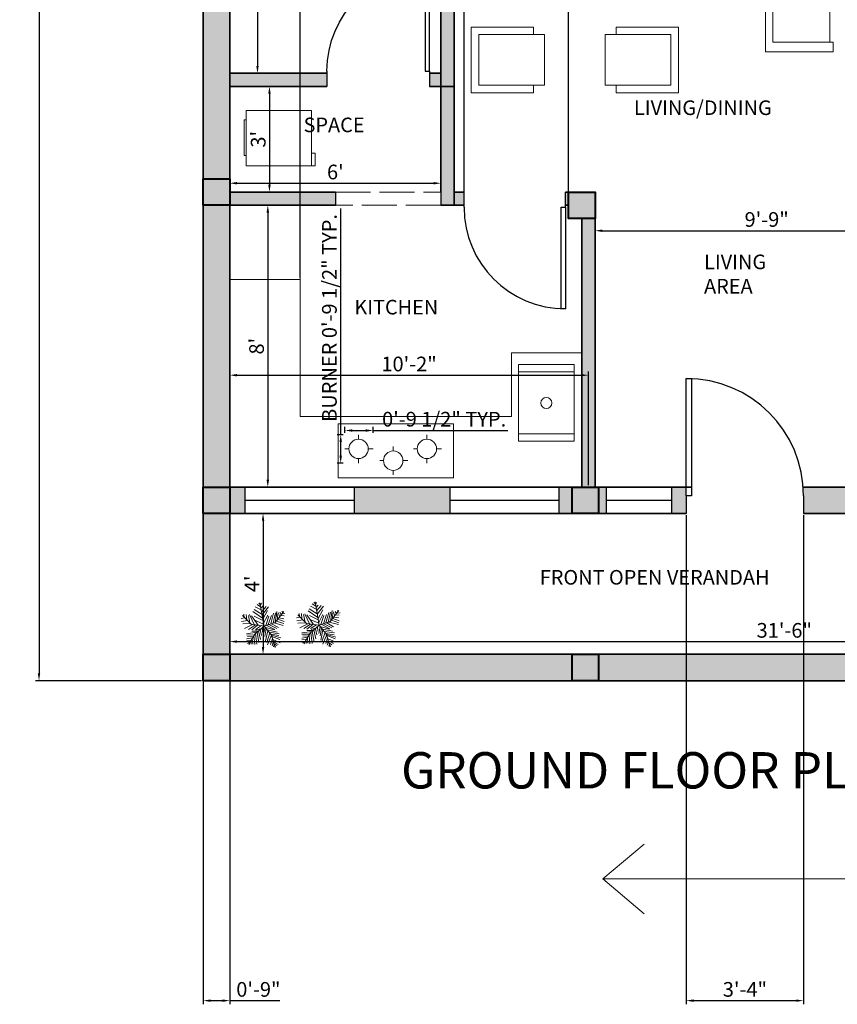
# Model space of a CAD drawing. Units: inches. Extents: x 1674 to 2231, y 1328 to 1959.
# Tile 1 of 6: x 1674 to 1952, y 1328 to 1664. Entities that reach past the tile are written whole.
import ezdxf

# ---------------------------------------------------------------- set-up
doc = ezdxf.new("R2010")
doc.units = ezdxf.units.IN
doc.linetypes.add('ACAD_ISO02W100', pattern=[15, 12, -3])
for name, color, linetype, lineweight in [('A-ANNO-DIMS', 113, 'Continuous', 18), ('A-ANNO-SYMB', 113, 'Continuous', 18), ('A-ANNO-TEXT', 113, 'Continuous', 18), ('A-AREA-IDEN', 113, 'Continuous', 18), ('A-COLS-PATT', 10, 'Continuous', 13), ('A-EQPM', 211, 'Continuous', 18), ('A-FLOR-CASE', 211, 'Continuous', 18), ('A-FLOR-FIXT', 211, 'Continuous', 18), ('A-GLAZ-HIDN', 181, 'ACAD_ISO02W100', 18), ('A-WALL-PATT', 140, 'Continuous', 13), ('COLUMN', 10, 'Continuous', 40), ('DOOR', 54, 'Continuous', 25), ('FUR', 211, 'Continuous', 18), ('TREE', 102, 'Continuous', 13), ('WALL', 7, 'Continuous', 35), ('WN', 181, 'Continuous', 25)]:
    doc.layers.add(name, color=color, linetype=linetype, lineweight=lineweight)
doc.styles.get("Standard").update_dxf_attribs({"font": 'arial.ttf'})
doc.dimstyles.new('ISO-25', dxfattribs={"dimtxt": 5, "dimasz": 2.5, "dimexe": 1.25, "dimexo": 0.625, "dimtad": 1, "dimdec": 0, "dimlunit": 4, "dimtxsty": 'Standard', "dimcen": 2.5, "dimadec": 0, "dimazin": 0, "dimtfac": 1, "dimtdec": 0, "dimtmove": 0, "dimatfit": 3, "dimfxl": 1, "dimarcsym": 0})

# ---------------------------------------------------------------- blocks, each defined once
blk = doc.blocks.new('*U2')
for p, q in [((0, 0), (0, -6)), ((40, 0), (40, -6))]:
    blk.add_line(p, q)
blk.add_lwpolyline([(0, 0), (0, 40), (1.75, 40), (1.75, 0)], close=True)
blk.add_arc((0, 0), 40, 0, 90)
blk = doc.blocks.new('*U8')
for p, q in [((-8.737, 47.138), (-17.069, 52.711)), ((-10.186, 53.64), (-13.084, 55.962)), ((0, 0), (-10.5, 57)), ((-9.099, 51.782), (-6.563, 55.962)), ((-7.65, 43.423), (-2.578, 49.46)), ((-31.5, 4.5), (-52.5, 25.5)), ((-48.585, 21.131), (-49.309, 29.026)), ((-43.513, 28.561), (-42.427, 15.558)), ((-38.442, 26.239), (-34.819, 7.663)), ((-35.544, 28.097), (-24.314, 3.947)), ((-14.533, 2.09), (-30.834, 25.31)), ((-3.665, 19.273), (-27.574, 35.527)), ((-5.114, 28.097), (-24.676, 40.636)), ((-7.288, 39.707), (-21.778, 46.673)), ((-5.839, 35.992), (4.667, 48.067)), ((-5.114, 27.632), (10.463, 46.673)), ((-2.941, 16.486), (8.652, 37.85)), ((-1.129, 6.734), (9.014, 26.704)), ((3.942, 1.625), (11.187, 24.381)), ((10.101, 3.483), (17.708, 26.239)), ((16.259, 5.805), (23.142, 31.348)), ((22.055, 7.198), (27.489, 32.277)), ((27, 9), (48, 36)), ((27.127, 9.056), (31.112, 35.992)), ((31.836, 30.883), (32.561, 16.486)), ((35.096, 32.741), (37.27, 22.524)), ((38.719, 34.134), (41.979, 28.561)), ((40.53, 25.775), (48.862, 24.846)), ((43.791, 29.954), (51.036, 30.883)), ((44.153, 36.456), (45.239, 32.741)), ((-47.498, 19.737), (-55.83, 18.344)), ((-40.615, 13.7), (-55.105, 10.913)), ((-33.37, 6.269), (-52.207, 5.34)), ((-28.299, 3.483), (-47.86, -5.805)), ((-21.416, 3.018), (-38.079, -8.128)), ((0, 0), (-31.5, 4.5)), ((-15.982, 2.09), (-30.11, -9.521)), ((-24.314, 23.917), (-2.941, 13.7)), ((0, 0), (-22.5, -19.5)), ((-6.563, 1.161), (-21.416, -8.128)), ((-20.691, 13.7), (-1.129, 4.876)), ((0, 0), (27, 9)), ((0, 0), (18, -22.5)), ((6.478, 1.625), (26.04, -8.592)), ((11.187, 3.483), (30.749, -5.805)), ((18.07, 5.805), (35.096, -3.483)), ((24.229, 7.663), (46.688, 1.625)), ((29.662, 12.307), (48.137, 6.269)), ((33.285, 16.486), (48.862, 10.913)), ((36.183, 19.737), (48.137, 17.88)), ((-17.431, -15.094), (-42.789, -18.809)), ((-24.314, -21.596), (-42.427, -22.06)), ((-22.5, -19.5), (-37.5, -45)), ((-15.257, -12.772), (-30.11, -12.772)), ((-25.038, -23.918), (-22.865, -45.281)), ((-20.691, -18.345), (-17.793, -44.352)), ((-6.563, -5.805), (-19.967, -9.985)), ((-17.069, -15.094), (-12.721, -40.172)), ((-13.446, -11.378), (-8.737, -32.741)), ((-9.461, -8.592), (-6.201, -23.453)), ((-4.752, -3.483), (-3.665, -14.629)), ((2.493, -3.019), (-1.491, -20.202)), ((1.769, -2.555), (24.229, -9.521)), ((5.029, -6.27), (2.131, -25.775)), ((9.014, -11.378), (3.58, -35.992)), ((14.085, -16.951), (6.478, -40.172)), ((7.565, -9.056), (32.198, -14.629)), ((18.07, -22.524), (8.289, -45.745)), ((12.274, -15.094), (36.907, -18.809)), ((16.259, -19.738), (36.183, -22.989)), ((18, -22.5), (27, -52.5)), ((18.433, -22.524), (40.53, -29.026)), ((-28.299, -29.026), (-42.789, -31.348)), ((-30.834, -34.135), (-42.427, -35.528)), ((-34.457, -39.708), (-40.978, -42.494)), ((-26.849, -26.24), (-40.253, -25.775)), ((-32.646, -36.921), (-31.921, -44.352)), ((-29.023, -30.884), (-27.936, -43.887)), ((20.244, -30.419), (15.897, -44.816)), ((19.157, -25.311), (38.719, -33.206)), ((22.78, -37.85), (19.519, -48.532)), ((21.331, -32.741), (39.081, -40.636)), ((22.78, -38.314), (34.372, -44.816)), ((24.591, -45.745), (23.142, -50.854)), ((24.591, -43.423), (30.749, -47.603)), ((26.764, -49.925), (28.213, -50.854))]:
    blk.add_line(p, q)
blk = doc.blocks.new('*D10')
at = {"layer": 'A-ANNO-DIMS', "color": 0, "lineweight": -2, "transparency": 16777216}
for p, q in [((1735.65, 1918.36), (1679.03, 1918.36)), ((1680.28, 1915.86), (1680.28, 1440.86)), ((1735.65, 1438.36), (1679.03, 1438.36))]:
    blk.add_line(p, q, dxfattribs=at)
at = {"layer": 'A-ANNO-DIMS', "color": 0, "lineweight": 100, "transparency": 16777216}
for points in [[(1679.86, 1915.86), (1680.69, 1915.86), (1680.28, 1918.36)], [(1679.86, 1440.86), (1680.69, 1440.86), (1680.28, 1438.36)]]:
    blk.add_solid(points, dxfattribs=at)
at = {"layer": 'Defpoints', "color": 0, "lineweight": 100, "transparency": 16777216}
for p in [(1736.27, 1918.36), (1680.28, 1438.36), (1736.27, 1438.36)]:
    blk.add_point(p, dxfattribs=at)
at = {"layer": 'A-ANNO-DIMS', "color": 0, "transparency": 16777216, "insert": (1677.1, 1678.36), "char_height": 5, "attachment_point": 5, "rotation": 90}
blk.add_mtext("40'", dxfattribs=at)
blk = doc.blocks.new('*D23')
at = {"layer": 'A-ANNO-DIMS', "color": 0, "lineweight": -2, "transparency": 16777216}
for p, q in [((1745.9, 1748.86), (1755.99, 1748.86)), ((1754.74, 1746.36), (1754.74, 1647.86)), ((1745.9, 1645.36), (1755.99, 1645.36))]:
    blk.add_line(p, q, dxfattribs=at)
at = {"layer": 'A-ANNO-DIMS', "color": 0, "lineweight": 100, "transparency": 16777216}
for points in [[(1754.32, 1746.36), (1755.15, 1746.36), (1754.74, 1748.86)], [(1754.32, 1647.86), (1755.15, 1647.86), (1754.74, 1645.36)]]:
    blk.add_solid(points, dxfattribs=at)
at = {"layer": 'Defpoints', "color": 0, "lineweight": 100, "transparency": 16777216}
for p in [(1745.27, 1748.86), (1745.27, 1645.36), (1754.74, 1645.36)]:
    blk.add_point(p, dxfattribs=at)
at = {"layer": 'A-ANNO-DIMS', "color": 0, "transparency": 16777216, "insert": (1751.56, 1697.11), "char_height": 5, "attachment_point": 5, "rotation": 90}
blk.add_mtext('8\'-8"', dxfattribs=at)
blk = doc.blocks.new('*D24')
at = {"layer": 'A-ANNO-DIMS', "color": 0, "lineweight": -2, "transparency": 16777216}
for p, q in [((1745.9, 1640.86), (1760.06, 1640.86)), ((1758.81, 1638.36), (1758.81, 1607.36)), ((1745.9, 1604.86), (1760.06, 1604.86))]:
    blk.add_line(p, q, dxfattribs=at)
at = {"layer": 'A-ANNO-DIMS', "color": 0, "lineweight": 100, "transparency": 16777216}
for points in [[(1758.39, 1638.36), (1759.23, 1638.36), (1758.81, 1640.86)], [(1758.39, 1607.36), (1759.23, 1607.36), (1758.81, 1604.86)]]:
    blk.add_solid(points, dxfattribs=at)
at = {"layer": 'Defpoints', "color": 0, "lineweight": 100, "transparency": 16777216}
for p in [(1745.27, 1640.86), (1745.27, 1604.86), (1758.81, 1604.86)]:
    blk.add_point(p, dxfattribs=at)
at = {"layer": 'A-ANNO-DIMS', "color": 0, "transparency": 16777216, "insert": (1755.63, 1622.86), "char_height": 5, "attachment_point": 5, "rotation": 90}
blk.add_mtext("3'", dxfattribs=at)
blk = doc.blocks.new('*D25')
at = {"layer": 'A-ANNO-DIMS', "color": 0, "lineweight": -2, "transparency": 16777216}
for p, q in [((1745.27, 1605.48), (1745.27, 1609.13)), ((1747.77, 1607.88), (1814.77, 1607.88)), ((1817.27, 1605.48), (1817.27, 1609.13))]:
    blk.add_line(p, q, dxfattribs=at)
at = {"layer": 'A-ANNO-DIMS', "color": 0, "lineweight": 100, "transparency": 16777216}
for points in [[(1747.77, 1608.3), (1747.77, 1607.46), (1745.27, 1607.88)], [(1814.77, 1608.3), (1814.77, 1607.46), (1817.27, 1607.88)]]:
    blk.add_solid(points, dxfattribs=at)
at = {"layer": 'Defpoints', "color": 0, "lineweight": 100, "transparency": 16777216}
for p in [(1817.27, 1607.88), (1745.27, 1604.86), (1817.27, 1604.86)]:
    blk.add_point(p, dxfattribs=at)
at = {"layer": 'A-ANNO-DIMS', "color": 0, "transparency": 16777216, "insert": (1781.27, 1611.06), "char_height": 5, "attachment_point": 5}
blk.add_mtext("6'", dxfattribs=at)
blk = doc.blocks.new('*D26')
at = {"layer": 'A-ANNO-DIMS', "color": 0, "lineweight": -2, "transparency": 16777216}
for p, q in [((1745.9, 1600.36), (1759.5, 1600.36)), ((1758.25, 1597.86), (1758.25, 1506.86)), ((1745.9, 1504.36), (1759.5, 1504.36))]:
    blk.add_line(p, q, dxfattribs=at)
at = {"layer": 'A-ANNO-DIMS', "color": 0, "lineweight": 100, "transparency": 16777216}
for points in [[(1757.83, 1597.86), (1758.67, 1597.86), (1758.25, 1600.36)], [(1757.83, 1506.86), (1758.67, 1506.86), (1758.25, 1504.36)]]:
    blk.add_solid(points, dxfattribs=at)
at = {"layer": 'Defpoints', "color": 0, "lineweight": 100, "transparency": 16777216}
for p in [(1745.27, 1600.36), (1745.27, 1504.36), (1758.25, 1504.36)]:
    blk.add_point(p, dxfattribs=at)
at = {"layer": 'A-ANNO-DIMS', "color": 0, "transparency": 16777216, "insert": (1755.07, 1552.36), "char_height": 5, "attachment_point": 5, "rotation": 90}
blk.add_mtext("8'", dxfattribs=at)
blk = doc.blocks.new('*D27')
at = {"layer": 'A-ANNO-DIMS', "color": 0, "lineweight": -2, "transparency": 16777216}
for p, q in [((1745.27, 1504.98), (1745.27, 1543.72)), ((1867.52, 1504.98), (1867.52, 1543.72)), ((1747.77, 1542.47), (1865.02, 1542.47))]:
    blk.add_line(p, q, dxfattribs=at)
at = {"layer": 'A-ANNO-DIMS', "color": 0, "lineweight": 100, "transparency": 16777216}
for points in [[(1747.77, 1542.88), (1747.77, 1542.05), (1745.27, 1542.47)], [(1865.02, 1542.88), (1865.02, 1542.05), (1867.52, 1542.47)]]:
    blk.add_solid(points, dxfattribs=at)
at = {"layer": 'Defpoints', "color": 0, "lineweight": 100, "transparency": 16777216}
for p in [(1867.52, 1542.47), (1745.27, 1504.36), (1867.52, 1504.36)]:
    blk.add_point(p, dxfattribs=at)
at = {"layer": 'A-ANNO-DIMS', "color": 0, "transparency": 16777216, "insert": (1806.4, 1545.64), "char_height": 5, "attachment_point": 5}
blk.add_mtext('10\'-2"', dxfattribs=at)
blk = doc.blocks.new('*D28')
at = {"layer": 'A-ANNO-DIMS', "color": 0, "lineweight": -2, "transparency": 16777216}
for p, q in [((1745.9, 1495.36), (1757.88, 1495.36)), ((1756.63, 1492.86), (1756.63, 1449.86)), ((1745.9, 1447.36), (1757.88, 1447.36))]:
    blk.add_line(p, q, dxfattribs=at)
at = {"layer": 'A-ANNO-DIMS', "color": 0, "lineweight": 100, "transparency": 16777216}
for points in [[(1756.22, 1492.86), (1757.05, 1492.86), (1756.63, 1495.36)], [(1756.22, 1449.86), (1757.05, 1449.86), (1756.63, 1447.36)]]:
    blk.add_solid(points, dxfattribs=at)
at = {"layer": 'Defpoints', "color": 0, "lineweight": 100, "transparency": 16777216}
for p in [(1745.27, 1495.36), (1745.27, 1447.36), (1756.63, 1447.36)]:
    blk.add_point(p, dxfattribs=at)
at = {"layer": 'A-ANNO-DIMS', "color": 0, "transparency": 16777216, "insert": (1753.51, 1471.36), "char_height": 5, "attachment_point": 5, "rotation": 90}
blk.add_mtext("4'", dxfattribs=at)
blk = doc.blocks.new('*D29')
at = {"layer": 'A-ANNO-DIMS', "color": 0, "lineweight": -2, "transparency": 16777216}
for p, q in [((1745.27, 1447.98), (1745.27, 1452.95)), ((2123.27, 1447.98), (2123.27, 1452.95)), ((1747.77, 1451.7), (2120.77, 1451.7))]:
    blk.add_line(p, q, dxfattribs=at)
at = {"layer": 'A-ANNO-DIMS', "color": 0, "lineweight": 100, "transparency": 16777216}
for points in [[(1747.77, 1452.12), (1747.77, 1451.28), (1745.27, 1451.7)], [(2120.77, 1452.12), (2120.77, 1451.28), (2123.27, 1451.7)]]:
    blk.add_solid(points, dxfattribs=at)
at = {"layer": 'Defpoints', "color": 0, "lineweight": 100, "transparency": 16777216}
for p in [(2123.27, 1451.7), (1745.27, 1447.36), (2123.27, 1447.36)]:
    blk.add_point(p, dxfattribs=at)
at = {"layer": 'A-ANNO-DIMS', "color": 0, "transparency": 16777216, "insert": (1934.27, 1454.88), "char_height": 5, "attachment_point": 5}
blk.add_mtext('31\'-6"', dxfattribs=at)
blk = doc.blocks.new('*D30')
at = {"layer": 'A-ANNO-DIMS', "color": 0, "lineweight": -2, "transparency": 16777216}
for p, q in [((1869.77, 1504.98), (1869.77, 1592.95)), ((1872.27, 1591.7), (1984.27, 1591.7)), ((1986.77, 1504.98), (1986.77, 1592.95))]:
    blk.add_line(p, q, dxfattribs=at)
at = {"layer": 'A-ANNO-DIMS', "color": 0, "lineweight": 100, "transparency": 16777216}
for points in [[(1872.27, 1592.11), (1872.27, 1591.28), (1869.77, 1591.7)], [(1984.27, 1592.11), (1984.27, 1591.28), (1986.77, 1591.7)]]:
    blk.add_solid(points, dxfattribs=at)
at = {"layer": 'Defpoints', "color": 0, "lineweight": 100, "transparency": 16777216}
for p in [(1986.77, 1591.7), (1869.77, 1504.36), (1986.77, 1504.36)]:
    blk.add_point(p, dxfattribs=at)
at = {"layer": 'A-ANNO-DIMS', "color": 0, "transparency": 16777216, "insert": (1928.27, 1594.88), "char_height": 5, "attachment_point": 5}
blk.add_mtext('9\'-9"', dxfattribs=at)
blk = doc.blocks.new('CHAIR-DINING')
for p, q in [((21.28, 22.31), (0, 22.31)), ((0, 22.31), (0, 0)), ((21.28, 19.89), (21.28, 22.31)), ((0, 0), (21.28, 0)), ((21.28, 0), (21.28, 2.58))]:
    blk.add_line(p, q)
blk.add_lwpolyline([(25.04, 19.89), (2.65, 19.89), (2.65, 2.58), (25.04, 2.58)], close=True)
blk = doc.blocks.new('ARROW-ROAD-DIRECTION')
for p, q in [((0, 11.86), (14.05, 23.72)), ((88.42, 11.86), (0, 11.86)), ((4.6, 11.86), (0, 11.86)), ((0, 11.86), (14.05, 0))]:
    blk.add_line(p, q)
blk = doc.blocks.new('COOKTOP-BURNER')
for p, q in [((4.62, 8.16), (4.62, 9.66)), ((1.32, 4.86), (0, 4.86)), ((7.93, 4.86), (9.61, 4.86)), ((4.62, 1.56), (4.62, 0))]:
    blk.add_line(p, q)
blk.add_circle((4.62, 4.86), 3.3)
blk = doc.blocks.new('*D44')
at = {"layer": 'A-ANNO-DIMS', "color": 0, "lineweight": -2, "transparency": 16777216}
for p, q in [((1783.1, 1522.17), (1783.1, 1599.27)), ((1783.92, 1522.17), (1781.85, 1522.17)), ((1783.1, 1515.01), (1783.1, 1519.67)), ((1783.92, 1512.51), (1781.85, 1512.51))]:
    blk.add_line(p, q, dxfattribs=at)
at = {"layer": 'A-ANNO-DIMS', "color": 0, "lineweight": 100, "transparency": 16777216}
for points in [[(1782.68, 1519.67), (1783.52, 1519.67), (1783.1, 1522.17)], [(1782.68, 1515.01), (1783.52, 1515.01), (1783.1, 1512.51)]]:
    blk.add_solid(points, dxfattribs=at)
at = {"layer": 'Defpoints', "color": 0, "lineweight": 100, "transparency": 16777216}
for p in [(1783.1, 1522.17), (1784.55, 1522.17), (1784.55, 1512.51)]:
    blk.add_point(p, dxfattribs=at)
at = {"layer": 'A-ANNO-DIMS', "color": 0, "transparency": 16777216, "insert": (1779.89, 1561.97), "char_height": 5, "attachment_point": 5, "rotation": 90}
blk.add_mtext('BURNER 0\'-9 1/2" TYP.', dxfattribs=at)
blk = doc.blocks.new('*D45')
at = {"layer": 'A-ANNO-DIMS', "color": 0, "lineweight": -2, "transparency": 16777216}
for p, q in [((1784.55, 1522.8), (1784.55, 1524.87)), ((1787.05, 1523.62), (1791.66, 1523.62)), ((1794.16, 1522.8), (1794.16, 1524.87)), ((1794.16, 1523.62), (1840.03, 1523.62))]:
    blk.add_line(p, q, dxfattribs=at)
at = {"layer": 'A-ANNO-DIMS', "color": 0, "lineweight": 100, "transparency": 16777216}
for points in [[(1787.05, 1524.04), (1787.05, 1523.21), (1784.55, 1523.62)], [(1791.66, 1524.04), (1791.66, 1523.21), (1794.16, 1523.62)]]:
    blk.add_solid(points, dxfattribs=at)
at = {"layer": 'Defpoints', "color": 0, "lineweight": 100, "transparency": 16777216}
for p in [(1794.16, 1523.62), (1784.55, 1522.17), (1794.16, 1522.17)]:
    blk.add_point(p, dxfattribs=at)
at = {"layer": 'A-ANNO-DIMS', "color": 0, "transparency": 16777216, "insert": (1818.35, 1526.83), "char_height": 5, "attachment_point": 5}
blk.add_mtext('0\'-9 1/2" TYP.', dxfattribs=at)
blk = doc.blocks.new('*D51')
at = {"layer": 'A-ANNO-DIMS', "color": 0, "lineweight": -2, "transparency": 16777216}
for p, q in [((1900.85, 1494.73), (1900.85, 1328.11)), ((1940.85, 1494.73), (1940.85, 1328.11)), ((1903.35, 1329.36), (1938.35, 1329.36))]:
    blk.add_line(p, q, dxfattribs=at)
at = {"layer": 'A-ANNO-DIMS', "color": 0, "lineweight": 100, "transparency": 16777216}
for points in [[(1903.35, 1329.77), (1903.35, 1328.94), (1900.85, 1329.36)], [(1938.35, 1329.77), (1938.35, 1328.94), (1940.85, 1329.36)]]:
    blk.add_solid(points, dxfattribs=at)
at = {"layer": 'Defpoints', "color": 0, "lineweight": 100, "transparency": 16777216}
for p in [(1900.85, 1495.36), (1940.85, 1495.36), (1940.85, 1329.36)]:
    blk.add_point(p, dxfattribs=at)
at = {"layer": 'A-ANNO-DIMS', "color": 0, "transparency": 16777216, "insert": (1920.85, 1332.54), "char_height": 5, "attachment_point": 5}
blk.add_mtext('3\'-4"', dxfattribs=at)
blk = doc.blocks.new('*D54')
at = {"layer": 'A-ANNO-DIMS', "color": 0, "lineweight": -2, "transparency": 16777216}
for p, q in [((1745.27, 1575.73), (1745.27, 1949.21)), ((1747.77, 1947.96), (1766.77, 1947.96)), ((1769.27, 1575.73), (1769.27, 1949.21))]:
    blk.add_line(p, q, dxfattribs=at)
at = {"layer": 'A-ANNO-DIMS', "color": 0, "lineweight": 100, "transparency": 16777216}
for points in [[(1747.77, 1948.37), (1747.77, 1947.54), (1745.27, 1947.96)], [(1766.77, 1948.37), (1766.77, 1947.54), (1769.27, 1947.96)]]:
    blk.add_solid(points, dxfattribs=at)
at = {"layer": 'Defpoints', "color": 0, "lineweight": 100, "transparency": 16777216}
for p in [(1769.27, 1947.96), (1745.27, 1575.1), (1769.27, 1575.1)]:
    blk.add_point(p, dxfattribs=at)
at = {"layer": 'A-ANNO-DIMS', "color": 0, "transparency": 16777216, "insert": (1757.27, 1951.13), "char_height": 5, "attachment_point": 5}
blk.add_mtext('2\'-0"', dxfattribs=at)
blk = doc.blocks.new('*D55')
at = {"layer": 'A-ANNO-DIMS', "color": 0, "lineweight": -2, "transparency": 16777216}
for p, q in [((1736.27, 1494.73), (1736.27, 1328.11)), ((1745.27, 1494.73), (1745.27, 1328.11)), ((1738.77, 1329.36), (1742.77, 1329.36)), ((1745.27, 1329.36), (1762.31, 1329.36))]:
    blk.add_line(p, q, dxfattribs=at)
at = {"layer": 'A-ANNO-DIMS', "color": 0, "lineweight": 100, "transparency": 16777216}
for points in [[(1738.77, 1329.77), (1738.77, 1328.94), (1736.27, 1329.36)], [(1742.77, 1329.77), (1742.77, 1328.94), (1745.27, 1329.36)]]:
    blk.add_solid(points, dxfattribs=at)
at = {"layer": 'Defpoints', "color": 0, "lineweight": 100, "transparency": 16777216}
for p in [(1736.27, 1495.36), (1745.27, 1495.36), (1745.27, 1329.36)]:
    blk.add_point(p, dxfattribs=at)
at = {"layer": 'A-ANNO-DIMS', "color": 0, "transparency": 16777216, "insert": (1755.04, 1332.54), "char_height": 5, "attachment_point": 5}
blk.add_mtext('0\'-9"', dxfattribs=at)
blk = doc.blocks.new('*D56')
at = {"layer": 'A-ANNO-DIMS', "color": 0, "lineweight": -2, "transparency": 16777216}
for p, q in [((1825.14, 1600.98), (1825.14, 1949.21)), ((1827.64, 1947.96), (1858.27, 1947.96)), ((1860.77, 1600.98), (1860.77, 1949.21))]:
    blk.add_line(p, q, dxfattribs=at)
at = {"layer": 'A-ANNO-DIMS', "color": 0, "lineweight": 100, "transparency": 16777216}
for points in [[(1827.64, 1948.37), (1827.64, 1947.54), (1825.14, 1947.96)], [(1858.27, 1948.37), (1858.27, 1947.54), (1860.77, 1947.96)]]:
    blk.add_solid(points, dxfattribs=at)
at = {"layer": 'Defpoints', "color": 0, "lineweight": 100, "transparency": 16777216}
for p in [(1860.77, 1947.96), (1825.14, 1600.36), (1860.77, 1600.36)]:
    blk.add_point(p, dxfattribs=at)
at = {"layer": 'A-ANNO-DIMS', "color": 0, "transparency": 16777216, "insert": (1842.96, 1951.17), "char_height": 5, "attachment_point": 5}
blk.add_mtext('2\'-11 1/2"', dxfattribs=at)

msp = doc.modelspace()

# ---------------------------------------------------------------- hatches: boundary and pattern name
at = {"layer": 'A-COLS-PATT'}
h = msp.add_hatch(color=256, dxfattribs=at)
h.dxf.hatch_style = 1
h.paths.add_polyline_path([(1745.27, 1918.36), (1736.27, 1918.36), (1736.27, 1909.36), (1745.27, 1909.36)])
h.paths.add_polyline_path([(1886.27, 1918.36), (1877.27, 1918.36), (1877.27, 1909.36), (1886.27, 1909.36)])
h.paths.add_polyline_path([(1995.77, 1918.36), (1986.77, 1918.36), (1986.77, 1909.36), (1995.77, 1909.36)])
h.paths.add_polyline_path([(2132.27, 1918.36), (2123.27, 1918.36), (2123.27, 1909.36), (2132.27, 1909.36)])
h.paths.add_polyline_path([(1745.27, 1757.86), (1736.27, 1757.86), (1736.27, 1748.86), (1745.27, 1748.86)])
h.paths.add_polyline_path([(1886.27, 1757.86), (1877.27, 1757.86), (1877.27, 1748.86), (1886.27, 1748.86)])
h.paths.add_polyline_path([(2132.27, 1757.81), (2123.27, 1757.81), (2123.27, 1748.81), (2132.27, 1748.81)])
h.paths.add_polyline_path([(1995.77, 1757.86), (1986.77, 1757.86), (1986.77, 1748.86), (1995.77, 1748.86)])
h.paths.add_polyline_path([(2132.27, 1625.36), (2123.27, 1625.36), (2123.27, 1616.36), (2132.27, 1616.36)])
h.paths.add_polyline_path([(1995.77, 1625.36), (1986.77, 1625.36), (1986.77, 1616.36), (1995.77, 1616.36)])
h.paths.add_polyline_path([(1869.77, 1604.86), (1860.77, 1604.86), (1860.77, 1595.86), (1869.77, 1595.86)])
h.paths.add_polyline_path([(1745.27, 1609.36), (1736.27, 1609.36), (1736.27, 1600.36), (1745.27, 1600.36)])
h.paths.add_polyline_path([(1745.27, 1504.36), (1736.27, 1504.36), (1736.27, 1495.36), (1745.27, 1495.36)])
h.paths.add_polyline_path([(1870.95, 1504.36), (1861.95, 1504.36), (1861.95, 1495.36), (1870.95, 1495.36)])
h.paths.add_polyline_path([(1995.77, 1504.36), (1986.77, 1504.36), (1986.77, 1495.36), (1995.77, 1495.36)])
h.paths.add_polyline_path([(1995.77, 1447.36), (1986.77, 1447.36), (1986.77, 1438.36), (1995.77, 1438.36)])
h.paths.add_polyline_path([(2132.27, 1447.36), (2123.27, 1447.36), (2123.27, 1438.36), (2132.27, 1438.36)])
h = msp.add_hatch(color=256, dxfattribs=at)
h.dxf.hatch_style = 1
h.paths.add_polyline_path([(1745.27, 1447.36), (1736.27, 1447.36), (1736.27, 1438.36), (1745.27, 1438.36)])
h.paths.add_polyline_path([(1870.95, 1447.36), (1861.95, 1447.36), (1861.95, 1438.36), (1870.95, 1438.36)])
at = {"layer": 'A-WALL-PATT'}
h = msp.add_hatch(color=256, dxfattribs=at)
h.dxf.hatch_style = 1
h.paths.add_polyline_path([(1877.27, 1918.36), (1745.27, 1918.36), (1745.27, 1909.36), (1877.27, 1909.36)])
h.paths.add_polyline_path([(1986.77, 1918.36), (1886.27, 1918.36), (1886.27, 1909.36), (1986.77, 1909.36)])
h.paths.add_polyline_path([(2123.27, 1918.36), (1995.77, 1918.36), (1995.77, 1909.36), (2123.27, 1909.36)])
h.paths.add_polyline_path([(1894.11, 1861.36), (1886.27, 1861.36), (1886.27, 1865.74), (1881.77, 1865.74), (1881.77, 1808), (1881.77, 1798.89), (1884.87, 1798.89, -0.017002), (1886.27, 1798.84), (1886.27, 1852.36), (1894.11, 1852.36)])
h.paths.add_polyline_path([(1952.87, 1861.36), (1919.24, 1861.36), (1919.24, 1852.36), (1952.87, 1852.36)])
h.paths.add_polyline_path([(1991.27, 1865.74), (1986.77, 1865.74), (1986.77, 1861.36), (1976.26, 1861.36), (1976.26, 1852.36), (1986.77, 1852.36), (1986.77, 1847.49), (1986.77, 1757.86), (1991.27, 1757.86), (1991.27, 1852.36)])
h.paths.add_polyline_path([(1986.77, 1816.36), (1938.77, 1816.36), (1938.77, 1813.86), (1986.77, 1813.86)])
h.paths.add_polyline_path([(1934.27, 1819.36), (1886.27, 1819.36), (1886.27, 1816.86), (1934.27, 1816.86)])
h.paths.add_polyline_path([(1938.77, 1852.36), (1934.27, 1852.36), (1934.27, 1753.36), (1934.27, 1748.86), (1938.77, 1748.86), (1938.77, 1753.36)])
h.paths.add_polyline_path([(1934.27, 1777.36), (1915.46, 1777.36), (1886.27, 1777.36), (1886.27, 1772.86), (1934.27, 1772.86)])
h.paths.add_polyline_path([(1986.77, 1753.36), (1967.96, 1753.36), (1961.77, 1753.36, -0.017002), (1961.81, 1751.95), (1961.81, 1748.86), (1986.77, 1748.86)])
h.paths.add_polyline_path([(2000.84, 1753.36), (1995.77, 1753.36), (1995.77, 1748.86), (2000.84, 1748.86)])
h.paths.add_polyline_path([(1941.17, 1751.95), (1941.17, 1753.36), (1938.77, 1753.36), (1938.77, 1748.86), (1941.17, 1748.86)])
h.paths.add_polyline_path([(1877.27, 1753.36), (1875.49, 1753.36), (1875.49, 1748.86), (1877.27, 1748.86)])
h.paths.add_polyline_path([(1745.27, 1909.36), (1736.27, 1909.36), (1736.27, 1757.86), (1745.27, 1757.86), (1745.27, 1773.01)])
h.paths.add_polyline_path([(1778.41, 1645.36), (1745.27, 1645.36), (1745.27, 1640.86), (1778.41, 1640.86)])
h.paths.add_polyline_path([(1821.77, 1645.36), (1821.77, 1668.45), (1817.27, 1668.45), (1817.27, 1645.36), (1817.27, 1640.86), (1821.77, 1640.86)])
h.paths.add_polyline_path([(1817.27, 1645.36), (1813.39, 1645.36), (1813.39, 1640.86), (1817.27, 1640.86)])
h.paths.add_polyline_path([(1821.77, 1640.86), (1817.27, 1640.86), (1817.27, 1604.86), (1817.27, 1600.36), (1821.77, 1600.36)])
h.paths.add_polyline_path([(1825.14, 1604.86), (1821.77, 1604.86), (1821.77, 1600.36), (1825.14, 1600.36)])
h.paths.add_polyline_path([(1781.27, 1604.86), (1745.27, 1604.86), (1745.27, 1600.36), (1781.27, 1600.36)])
h = msp.add_hatch(color=256, dxfattribs=at)
h.dxf.hatch_style = 1
h.paths.add_polyline_path([(2132.27, 1909.36), (2123.27, 1909.36), (2123.27, 1757.81), (2132.27, 1757.81)], flags=17)
h.paths.add_polyline_path([(2123.27, 1753.36), (2040.84, 1753.36), (2040.84, 1748.86), (2123.27, 1748.86)], flags=17)
h.paths.add_polyline_path([(1840.51, 1753.36), (1745.27, 1753.36), (1745.27, 1748.86), (1817.27, 1748.86), (1840.51, 1748.86)], flags=17)
h.paths.add_polyline_path([(1745.27, 1748.86), (1736.27, 1748.86), (1736.27, 1609.36), (1745.27, 1609.36), (1745.27, 1640.86)], flags=17)
h.paths.add_polyline_path([(1745.27, 1600.36), (1736.27, 1600.36), (1736.27, 1504.36), (1745.27, 1504.36)], flags=17)
h.paths.add_polyline_path([(1745.27, 1495.36), (1736.27, 1495.36), (1736.27, 1447.36), (1745.27, 1447.36)], flags=17)
h.paths.add_polyline_path([(1820.35, 1504.36), (1787.69, 1504.36), (1787.69, 1495.36), (1820.35, 1495.36)], flags=17)
h.paths.add_polyline_path([(1750.58, 1504.36), (1745.27, 1504.36), (1745.27, 1495.36), (1750.58, 1495.36)], flags=17)
h.paths.add_polyline_path([(1861.95, 1504.36), (1857.47, 1504.36), (1857.47, 1495.36), (1861.95, 1495.36)], flags=17)
h.paths.add_polyline_path([(1873.66, 1504.36), (1870.95, 1504.36), (1870.95, 1495.36), (1873.66, 1495.36)], flags=17)
h.paths.add_polyline_path([(1900.85, 1501.36), (1900.85, 1504.36), (1895.88, 1504.36), (1895.88, 1495.36), (1900.85, 1495.36)], flags=17)
h.paths.add_polyline_path([(1869.77, 1595.86), (1865.27, 1595.86), (1865.27, 1504.36), (1869.77, 1504.36)], flags=17)
h.paths.add_polyline_path([(1958.26, 1504.36), (1940.74, 1504.36, -0.01877), (1940.85, 1501.36), (1940.85, 1495.36), (1958.26, 1495.36)], flags=17)
h.paths.add_polyline_path([(1995.77, 1531.51), (1986.77, 1531.51), (1986.77, 1504.36), (1995.77, 1504.36)], flags=17)
h.paths.add_polyline_path([(1986.77, 1504.36), (1980.49, 1504.36), (1980.49, 1495.36), (1986.77, 1495.36)], flags=17)
h.paths.add_polyline_path([(1995.77, 1616.36), (1986.77, 1616.36), (1986.77, 1585.02), (1995.77, 1585.02)], flags=17)
h.paths.add_polyline_path([(2000.1, 1620.86), (1995.77, 1620.86), (1995.77, 1616.36), (2000.1, 1616.36)], flags=17)
h.paths.add_polyline_path([(2053.57, 1620.86), (2040.1, 1620.86), (2040.1, 1616.36), (2053.57, 1616.36)], flags=17)
h.paths.add_polyline_path([(2123.27, 1620.86), (2109.12, 1620.86), (2109.12, 1616.36), (2123.27, 1616.36)], flags=17)
h.paths.add_polyline_path([(2132.27, 1616.36), (2123.27, 1616.36), (2123.27, 1447.36), (2132.27, 1447.36)], flags=17)
h.paths.add_polyline_path([(1986.77, 1447.36), (1870.95, 1447.36), (1870.95, 1438.36), (1986.77, 1438.36)])
h.paths.add_polyline_path([(1861.95, 1447.36), (1745.27, 1447.36), (1745.27, 1438.36), (1861.95, 1438.36)])
h.paths.add_polyline_path([(2132.27, 1918.36), (1736.27, 1918.36), (1736.27, 1504.36), (1745.27, 1504.36), (1745.27, 1600.36), (1745.27, 1909.36), (2123.27, 1909.36), (2123.27, 1447.36), (2132.27, 1447.36)])
h = msp.add_hatch(color=256, dxfattribs=at)
h.dxf.hatch_style = 1
h.paths.add_polyline_path([(1745.27, 1600.36), (1736.27, 1600.36), (1736.27, 1504.36), (1745.27, 1504.36)])
h.paths.add_polyline_path([(1745.27, 1748.86), (1736.27, 1748.86), (1736.27, 1609.36), (1745.27, 1609.36), (1745.27, 1640.86)])
h.paths.add_polyline_path([(1821.77, 1748.86), (1817.27, 1748.86), (1817.27, 1723.23), (1821.77, 1723.23)])
h = msp.add_hatch(color=256, dxfattribs=at)
h.dxf.hatch_style = 1
h.paths.add_polyline_path([(1860.77, 1604.86), (1859.69, 1604.86), (1859.69, 1600.36), (1860.77, 1600.36)])

# ---------------------------------------------------------------- linework, layer by layer
at = {"layer": 'A-EQPM'}
for points in [[(1750.89, 1613.84), (1773.12, 1613.84), (1773.12, 1632.67), (1750.89, 1632.67)], [(1750.89, 1617.35), (1750.19, 1617.35), (1750.19, 1629.54), (1750.89, 1629.54)], [(1773.12, 1613.84), (1774.35, 1613.84), (1774.35, 1618.11), (1773.12, 1618.11)], [(1782.24, 1525.86), (1821.49, 1525.86), (1821.49, 1507.55), (1782.24, 1507.55)]]:
    msp.add_lwpolyline(points, close=True, dxfattribs=at)
at = {"layer": 'A-FLOR-CASE'}
for p, q in [((1745.27, 1600.36), (1769.27, 1600.36)), ((1769.27, 1600.36), (1769.27, 1528.36)), ((1865.27, 1550.11), (1841.27, 1550.11)), ((1841.27, 1550.11), (1841.27, 1528.36)), ((1841.27, 1528.36), (1769.27, 1528.36))]:
    msp.add_line(p, q, dxfattribs=at)
msp.add_lwpolyline([(1745.27, 1600.36), (1769.27, 1600.36), (1769.27, 1575.1), (1745.27, 1575.1)], close=True, dxfattribs=at)
at = {"layer": 'A-FLOR-FIXT'}
for p, q in [((1843.74, 1543.6), (1862.66, 1543.6)), ((1843.74, 1522.51), (1862.66, 1522.51))]:
    msp.add_line(p, q, dxfattribs=at)
msp.add_lwpolyline([(1843.74, 1546.09), (1862.66, 1546.09), (1862.66, 1519.94), (1843.74, 1519.94)], close=True, dxfattribs=at)
msp.add_circle((1853.2, 1533.01), 1.89, dxfattribs=at)
at = {"layer": 'A-GLAZ-HIDN'}
msp.add_lwpolyline([(1817.27, 1600.36), (1781.27, 1600.36), (1781.27, 1604.86), (1817.27, 1604.86)], close=True, dxfattribs=at)
at = {"layer": 'COLUMN'}
for points in [[(1736.27, 1609.36), (1745.27, 1609.36), (1745.27, 1600.36), (1736.27, 1600.36)], [(1860.77, 1604.86), (1869.77, 1604.86), (1869.77, 1595.86), (1860.77, 1595.86)], [(1736.27, 1504.36), (1745.27, 1504.36), (1745.27, 1495.36), (1736.27, 1495.36)], [(1861.95, 1504.36), (1870.95, 1504.36), (1870.95, 1495.36), (1861.95, 1495.36)], [(1736.27, 1447.36), (1745.27, 1447.36), (1745.27, 1438.36), (1736.27, 1438.36)], [(1861.95, 1447.36), (1870.95, 1447.36), (1870.95, 1438.36), (1861.95, 1438.36)]]:
    msp.add_lwpolyline(points, close=True, dxfattribs=at)
at = {"layer": 'FUR'}
for p, q in [((1927.85, 1652.61), (1927.85, 1720.04)), ((1949.77, 1655.93), (1950.89, 1655.93)), ((1950.89, 1655.93), (1950.89, 1652.61)), ((1950.89, 1652.61), (1927.85, 1652.61))]:
    msp.add_line(p, q, dxfattribs=at)
msp.add_lwpolyline([(1930.34, 1717.22), (1949.77, 1717.22), (1949.77, 1655.93), (1930.34, 1655.93)], close=True, dxfattribs=at)
at = {"layer": 'WALL'}
for p, q in [((1736.27, 1438.36), (1736.27, 1918.36)), ((1817.27, 1748.86), (1817.27, 1645.36)), ((1821.77, 1748.86), (1821.77, 1640.86)), ((1778.41, 1645.36), (1745.27, 1645.36)), ((1817.27, 1645.36), (1813.39, 1645.36)), ((1817.27, 1604.86), (1817.27, 1645.36)), ((1821.77, 1600.36), (1821.77, 1645.36)), ((1745.27, 1640.86), (1745.27, 1604.86)), ((1778.41, 1640.86), (1745.27, 1640.86)), ((1821.77, 1640.86), (1813.39, 1640.86)), ((1745.27, 1604.86), (1781.27, 1604.86)), ((1825.14, 1604.86), (1821.77, 1604.86)), ((1869.77, 1604.86), (1859.69, 1604.86)), ((1869.77, 1504.36), (1869.77, 1604.86)), ((1745.27, 1600.36), (1781.27, 1600.36)), ((1745.27, 1600.36), (1745.27, 1504.36)), ((1817.27, 1600.36), (1821.77, 1600.36)), ((1825.14, 1600.36), (1821.77, 1600.36)), ((1860.77, 1600.36), (1859.69, 1600.36)), ((1865.27, 1504.36), (1865.27, 1595.86)), ((1745.27, 1504.36), (1865.27, 1504.36)), ((1865.27, 1504.36), (1869.77, 1504.36)), ((1869.77, 1504.36), (1902.6, 1504.36)), ((1940.74, 1504.36), (1986.77, 1504.36)), ((1745.27, 1495.36), (1869.77, 1495.36)), ((1869.77, 1495.36), (1900.85, 1495.36)), ((1940.85, 1495.36), (1995.77, 1495.36)), ((1995.77, 1438.36), (1736.27, 1438.36))]:
    msp.add_line(p, q, dxfattribs=at)
for points in [[(1995.77, 1438.36), (1736.27, 1438.36), (1736.27, 1918.36), (2132.27, 1918.36), (2132.27, 1438.36), (2123.27, 1438.36)], [(1995.77, 1447.36), (1745.27, 1447.36), (1745.27, 1909.36), (2123.27, 1909.36), (2123.27, 1447.36)]]:
    msp.add_lwpolyline(points, dxfattribs=at)
at = {"layer": 'WN'}
for p, q in [((1781.27, 1604.86), (1781.27, 1600.36)), ((1817.27, 1604.86), (1817.27, 1600.36)), ((1750.58, 1499.86), (1787.69, 1499.86)), ((1820.35, 1499.86), (1857.47, 1499.86)), ((1873.66, 1499.86), (1895.88, 1499.86))]:
    msp.add_line(p, q, dxfattribs=at)
for points in [[(1750.58, 1504.36), (1787.69, 1504.36), (1787.69, 1495.36), (1750.58, 1495.36)], [(1820.35, 1504.36), (1857.47, 1504.36), (1857.47, 1495.36), (1820.35, 1495.36)], [(1873.66, 1504.36), (1895.88, 1504.36), (1895.88, 1495.36), (1873.66, 1495.36)]]:
    msp.add_lwpolyline(points, close=True, dxfattribs=at)

# ---------------------------------------------------------------- block references
at = {"layer": 'A-ANNO-SYMB'}
msp.add_blockref('ARROW-ROAD-DIRECTION', (1872.46, 1358.96), dxfattribs=at)
at = {"layer": 'A-EQPM'}
for p in [(1784.55, 1512.51), (1807.85, 1512.51), (1796.38, 1508.49)]:
    msp.add_blockref('COOKTOP-BURNER', p, dxfattribs=at)
at = {"layer": 'DOOR', "xscale": -0.8744829560094038, "yscale": 0.8744829560094038, "zscale": 0.8744829560094038}
msp.add_blockref('*U2', (1813.39, 1646.1), dxfattribs=at)
at = {"layer": 'DOOR', "xscale": 0.863878905869771, "yscale": 0.863878905869771, "zscale": 0.863878905869771, "rotation": 180}
msp.add_blockref('*U2', (1859.69, 1599.67), dxfattribs=at)
at = {"layer": 'DOOR'}
msp.add_blockref('*U2', (1900.85, 1501.36), dxfattribs=at)
at = {"layer": 'FUR'}
msp.add_blockref('CHAIR-DINING', (1827.55, 1638.72), dxfattribs=at)
at = {"layer": 'FUR', "extrusion": (0, 0, -1), "zscale": -1}
msp.add_blockref('CHAIR-DINING', (-1898.25, 1638.72), dxfattribs=at)
at = {"layer": 'TREE', "xscale": 0.1393019906957703, "yscale": 0.1393019906957703, "zscale": 0.1393019906957703}
for p in [(1756.99, 1456.99), (1775.8, 1457.25)]:
    msp.add_blockref('*U8', p, dxfattribs=at)

# ---------------------------------------------------------------- texts
at = {"layer": 'A-ANNO-TEXT', "insert": (1803.67, 1414.03), "char_height": 12.3835, "attachment_point": 1}
msp.add_mtext_dynamic_manual_height_columns('GROUND FLOOR PLAN', width=223.3864, gutter_width=61.92, heights=[0], dxfattribs=at)
at = {"layer": 'A-AREA-IDEN', "attachment_point": 1}
for s, insert, char_height in [('LIVING/DINING', (1883.05, 1636.1), 4.9732), ('SPACE', (1770.44, 1630.24), 4.973), ('LIVING\\PAREA', (1906.93, 1583.57), 4.973), ('KITCHEN', (1787.74, 1568.15), 4.973), ('FRONT OPEN VERANDAH', (1850.94, 1476.09), 4.9732)]:
    msp.add_mtext_dynamic_manual_height_columns(s, width=89.7127, gutter_width=24.87, heights=[0], dxfattribs=dict(at, insert=insert, char_height=char_height))

# ---------------------------------------------------------------- dimensions: what is measured, and where the dimension line sits
at = {"layer": 'A-ANNO-DIMS'}
for base, p1, p2, override, picture, middle in [((1860.77, 1947.96), (1825.14, 1600.36), (1860.77, 1600.36), {"dimdec": 1, "dimlfac": 1, "dimrnd": 0, "dimzin": 1, "dimdsep": 46, "dimlunit": 4, "dimfrac": 2}, '*D56', (1842.96, 1951.17)), ((1769.27, 1947.96), (1745.27, 1575.1), (1769.27, 1575.1), {"dimdec": 1, "dimlfac": 1, "dimrnd": 0, "dimzin": 1, "dimdsep": 46, "dimlunit": 4, "dimfrac": 2}, '*D54', (1757.27, 1951.13)), ((1817.27, 1607.88), (1745.27, 1604.86), (1817.27, 1604.86), {"dimclrd": 0, "dimclre": 0, "dimclrt": 0}, '*D25', (1781.27, 1611.06)), ((1986.77, 1591.7), (1869.77, 1504.36), (1986.77, 1504.36), {"dimclrd": 0, "dimclre": 0, "dimclrt": 0}, '*D30', (1928.27, 1594.88)), ((1867.52, 1542.47), (1745.27, 1504.36), (1867.52, 1504.36), {"dimclrd": 0, "dimclre": 0, "dimclrt": 0}, '*D27', (1806.4, 1545.64)), ((1745.27, 1329.36), (1736.27, 1495.36), (1745.27, 1495.36), {"dimdec": 1, "dimlfac": 1, "dimrnd": 0, "dimzin": 1, "dimdsep": 46, "dimlunit": 4, "dimfrac": 2}, '*D55', (1755.04, 1332.54)), ((1940.85, 1329.36), (1900.85, 1495.36), (1940.85, 1495.36), {"dimdec": 1, "dimlfac": 1, "dimrnd": 0, "dimzin": 1, "dimdsep": 46, "dimlunit": 4, "dimfrac": 2}, '*D51', (1920.85, 1332.54)), ((2123.27, 1451.7), (1745.27, 1447.36), (2123.27, 1447.36), {"dimclrd": 0, "dimclre": 0, "dimclrt": 0}, '*D29', (1934.27, 1454.88))]:
    dim = msp.add_linear_dim(base=base, p1=p1, p2=p2, dimstyle='ISO-25', override=override, dxfattribs=at)
    dim.commit()
    dim.dimension.update_dxf_attribs({"geometry": picture, "text_midpoint": middle})
for base, p1, p2, picture, middle in [((1680.28, 1438.36), (1736.27, 1918.36), (1736.27, 1438.36), '*D10', (1677.1, 1678.36)), ((1754.73763243, 1645.35548105), (1745.27109151, 1748.85548105), (1745.27109151, 1645.35548105), '*D23', (1751.55976749, 1697.10548105)), ((1758.81, 1604.86), (1745.27, 1640.86), (1745.27, 1604.86), '*D24', (1755.63, 1622.86)), ((1758.25, 1504.36), (1745.27, 1600.36), (1745.27, 1504.36), '*D26', (1755.07, 1552.36)), ((1756.63, 1447.36), (1745.27, 1495.36), (1745.27, 1447.36), '*D28', (1753.51, 1471.36))]:
    dim = msp.add_linear_dim(base=base, p1=p1, p2=p2, angle=90, dimstyle='ISO-25', override={"dimclrd": 0, "dimclre": 0, "dimclrt": 0}, dxfattribs=at)
    dim.commit()
    dim.dimension.update_dxf_attribs({"geometry": picture, "text_midpoint": middle})
dim = msp.add_linear_dim(base=(1783.1, 1522.17), p1=(1784.55, 1512.51), p2=(1784.55, 1522.17), angle=90, text='BURNER <> TYP.', dimstyle='ISO-25', override={"dimdec": 1, "dimlfac": 1, "dimrnd": 0, "dimzin": 1, "dimdsep": 46, "dimlunit": 4, "dimfrac": 2}, dxfattribs=at)
dim.commit()
dim.dimension.update_dxf_attribs({"geometry": '*D44', "text_midpoint": (1779.89, 1561.97)})
dim = msp.add_linear_dim(base=(1794.16, 1523.62), p1=(1784.55, 1522.17), p2=(1794.16, 1522.17), text='<> TYP.', dimstyle='ISO-25', override={"dimdec": 1, "dimlfac": 1, "dimrnd": 0, "dimzin": 1, "dimdsep": 46, "dimlunit": 4, "dimfrac": 2}, dxfattribs=at)
dim.commit()
dim.dimension.update_dxf_attribs({"geometry": '*D45', "text_midpoint": (1818.35, 1526.83)})

doc.saveas('drawing.dxf')
